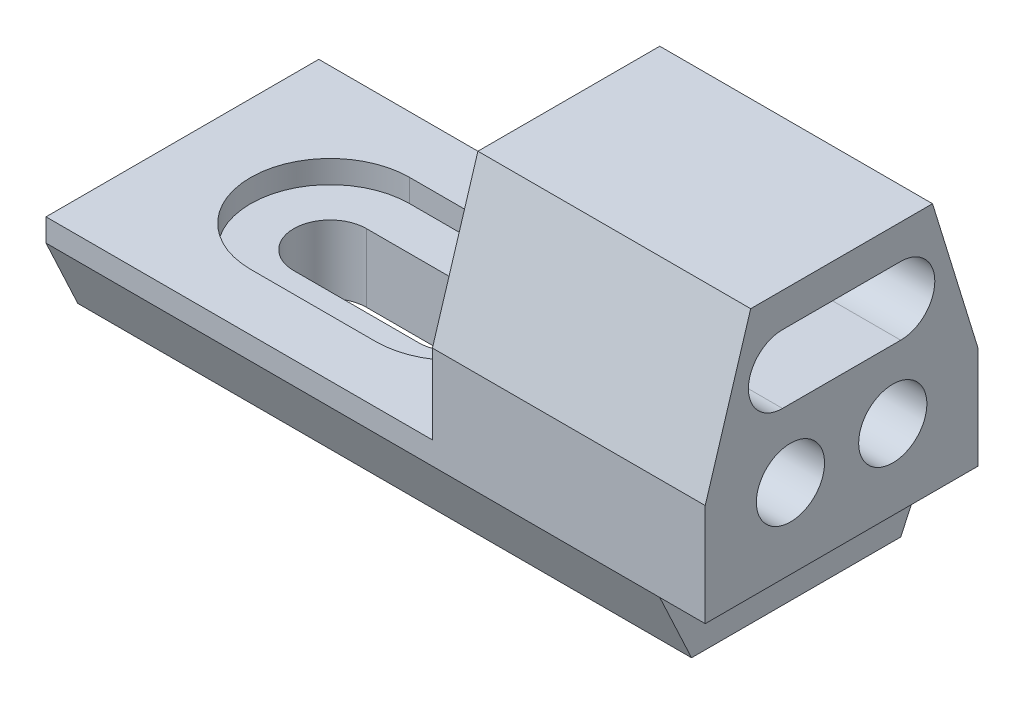
ISO-10303-21;
HEADER;
FILE_DESCRIPTION(('STEP AP214'),'2;1');
FILE_NAME('part.step','',(''),(''),'','','');
FILE_SCHEMA(('AUTOMOTIVE_DESIGN { 1 0 10303 214 1 1 1 1 }'));
ENDSEC;
DATA;
#1=APPLICATION_CONTEXT('core data for automotive mechanical design processes');
#2=APPLICATION_PROTOCOL_DEFINITION('international standard','automotive_design',2000,#1);
#3=PRODUCT_CONTEXT('',#1,'mechanical');
#4=PRODUCT('Part','Part','',(#3));
#5=PRODUCT_RELATED_PRODUCT_CATEGORY('part','',(#4));
#6=PRODUCT_DEFINITION_FORMATION('','',#4);
#7=PRODUCT_DEFINITION_CONTEXT('part definition',#1,'design');
#8=PRODUCT_DEFINITION('design','',#6,#7);
#9=PRODUCT_DEFINITION_SHAPE('','',#8);
#10=(LENGTH_UNIT() NAMED_UNIT(*) SI_UNIT(.MILLI.,.METRE.));
#11=(NAMED_UNIT(*) PLANE_ANGLE_UNIT() SI_UNIT($,.RADIAN.));
#12=(NAMED_UNIT(*) SI_UNIT($,.STERADIAN.) SOLID_ANGLE_UNIT());
#13=UNCERTAINTY_MEASURE_WITH_UNIT(LENGTH_MEASURE(1.E-05),#10,'distance_accuracy_value','');
#14=(GEOMETRIC_REPRESENTATION_CONTEXT(3) GLOBAL_UNCERTAINTY_ASSIGNED_CONTEXT((#13)) GLOBAL_UNIT_ASSIGNED_CONTEXT((#10,
#11,#12)) REPRESENTATION_CONTEXT('',''));
#15=CARTESIAN_POINT('',(0.,0.,0.));
#16=DIRECTION('',(0.,0.,1.));
#17=DIRECTION('',(1.,0.,0.));
#18=AXIS2_PLACEMENT_3D('',#15,#16,#17);
#19=CARTESIAN_POINT('',(0.,10.,0.));
#20=DIRECTION('',(0.,1.,0.));
#21=DIRECTION('',(0.,0.,1.));
#22=AXIS2_PLACEMENT_3D('',#19,#20,#21);
#23=PLANE('',#22);
#24=CARTESIAN_POINT('',(-80.,10.,0.));
#25=DIRECTION('',(0.,1.,0.));
#26=DIRECTION('',(0.,0.,1.));
#27=AXIS2_PLACEMENT_3D('',#24,#25,#26);
#28=CIRCLE('',#27,35.);
#29=CARTESIAN_POINT('',(-80.,10.,-35.));
#30=VERTEX_POINT('',#29);
#31=CARTESIAN_POINT('',(-80.,10.,35.));
#32=VERTEX_POINT('',#31);
#33=EDGE_CURVE('E222',#30,#32,#28,.T.);
#34=ORIENTED_EDGE('',*,*,#33,.F.);
#35=DIRECTION('',(-1.,0.,0.));
#36=VECTOR('',#35,1.);
#37=CARTESIAN_POINT('',(-80.,10.,-35.));
#38=LINE('',#37,#36);
#39=CARTESIAN_POINT('',(-25.,10.,-35.));
#40=VERTEX_POINT('',#39);
#41=EDGE_CURVE('E228',#40,#30,#38,.T.);
#42=ORIENTED_EDGE('',*,*,#41,.F.);
#43=CARTESIAN_POINT('',(-25.,10.,0.));
#44=DIRECTION('',(0.,1.,0.));
#45=DIRECTION('',(0.,0.,1.));
#46=AXIS2_PLACEMENT_3D('',#43,#44,#45);
#47=CIRCLE('',#46,35.);
#48=CARTESIAN_POINT('',(-25.,10.,35.));
#49=VERTEX_POINT('',#48);
#50=EDGE_CURVE('E244',#49,#40,#47,.T.);
#51=ORIENTED_EDGE('',*,*,#50,.F.);
#52=DIRECTION('',(1.,0.,0.));
#53=VECTOR('',#52,1.);
#54=CARTESIAN_POINT('',(-80.,10.,35.));
#55=LINE('',#54,#53);
#56=EDGE_CURVE('E238',#32,#49,#55,.T.);
#57=ORIENTED_EDGE('',*,*,#56,.F.);
#58=EDGE_LOOP('',(#34,#42,#51,#57));
#59=FACE_BOUND('',#58,.T.);
#60=DIRECTION('',(1.,0.,0.));
#61=VECTOR('',#60,1.);
#62=CARTESIAN_POINT('',(-145.,10.,60.));
#63=LINE('',#62,#61);
#64=CARTESIAN_POINT('',(-145.,10.,60.));
#65=VERTEX_POINT('',#64);
#66=CARTESIAN_POINT('',(25.,10.,60.));
#67=VERTEX_POINT('',#66);
#68=EDGE_CURVE('E366',#65,#67,#63,.T.);
#69=ORIENTED_EDGE('',*,*,#68,.T.);
#70=DIRECTION('',(0.,0.,-1.));
#71=VECTOR('',#70,1.);
#72=CARTESIAN_POINT('',(25.,10.,60.));
#73=LINE('',#72,#71);
#74=CARTESIAN_POINT('',(25.,10.,-60.));
#75=VERTEX_POINT('',#74);
#76=EDGE_CURVE('E312',#67,#75,#73,.T.);
#77=ORIENTED_EDGE('',*,*,#76,.T.);
#78=DIRECTION('',(-1.,0.,0.));
#79=VECTOR('',#78,1.);
#80=CARTESIAN_POINT('',(145.,10.,-60.));
#81=LINE('',#80,#79);
#82=CARTESIAN_POINT('',(-145.,10.,-60.));
#83=VERTEX_POINT('',#82);
#84=EDGE_CURVE('E361',#75,#83,#81,.T.);
#85=ORIENTED_EDGE('',*,*,#84,.T.);
#86=DIRECTION('',(0.,0.,1.));
#87=VECTOR('',#86,1.);
#88=CARTESIAN_POINT('',(-145.,10.,-60.));
#89=LINE('',#88,#87);
#90=EDGE_CURVE('E364',#83,#65,#89,.T.);
#91=ORIENTED_EDGE('',*,*,#90,.T.);
#92=EDGE_LOOP('',(#69,#77,#85,#91));
#93=FACE_BOUND('',#92,.T.);
#94=ADVANCED_FACE('F41',(#59,#93),#23,.T.);
#95=CARTESIAN_POINT('',(145.,10.,0.));
#96=DIRECTION('',(-1.,0.,0.));
#97=DIRECTION('',(0.,0.,1.));
#98=AXIS2_PLACEMENT_3D('',#95,#96,#97);
#99=PLANE('',#98);
#100=DIRECTION('',(0.,0.,-1.));
#101=VECTOR('',#100,1.);
#102=CARTESIAN_POINT('',(145.,95.,0.));
#103=LINE('',#102,#101);
#104=CARTESIAN_POINT('',(145.,95.,26.));
#105=VERTEX_POINT('',#104);
#106=CARTESIAN_POINT('',(145.,95.,-26.));
#107=VERTEX_POINT('',#106);
#108=EDGE_CURVE('E294',#105,#107,#103,.T.);
#109=ORIENTED_EDGE('',*,*,#108,.T.);
#110=CARTESIAN_POINT('',(145.,80.,-26.));
#111=DIRECTION('',(-1.,0.,0.));
#112=DIRECTION('',(0.,0.,1.));
#113=AXIS2_PLACEMENT_3D('',#110,#111,#112);
#114=CIRCLE('',#113,15.);
#115=CARTESIAN_POINT('',(145.,65.,-26.));
#116=VERTEX_POINT('',#115);
#117=EDGE_CURVE('E297',#107,#116,#114,.T.);
#118=ORIENTED_EDGE('',*,*,#117,.T.);
#119=DIRECTION('',(0.,0.,1.));
#120=VECTOR('',#119,1.);
#121=CARTESIAN_POINT('',(145.,65.,0.));
#122=LINE('',#121,#120);
#123=CARTESIAN_POINT('',(145.,65.,26.));
#124=VERTEX_POINT('',#123);
#125=EDGE_CURVE('E287',#116,#124,#122,.T.);
#126=ORIENTED_EDGE('',*,*,#125,.T.);
#127=CARTESIAN_POINT('',(145.,80.,26.));
#128=DIRECTION('',(-1.,0.,0.));
#129=DIRECTION('',(0.,0.,1.));
#130=AXIS2_PLACEMENT_3D('',#127,#128,#129);
#131=CIRCLE('',#130,15.);
#132=EDGE_CURVE('E292',#124,#105,#131,.T.);
#133=ORIENTED_EDGE('',*,*,#132,.T.);
#134=EDGE_LOOP('',(#109,#118,#126,#133));
#135=FACE_BOUND('',#134,.T.);
#136=CARTESIAN_POINT('',(145.,35.,22.5));
#137=DIRECTION('',(-1.,0.,0.));
#138=DIRECTION('',(0.,0.,1.));
#139=AXIS2_PLACEMENT_3D('',#136,#137,#138);
#140=CIRCLE('',#139,15.);
#141=CARTESIAN_POINT('',(145.,35.,37.5));
#142=VERTEX_POINT('',#141);
#143=EDGE_CURVE('E285',#142,#142,#140,.T.);
#144=ORIENTED_EDGE('',*,*,#143,.T.);
#145=EDGE_LOOP('',(#144));
#146=FACE_BOUND('',#145,.T.);
#147=CARTESIAN_POINT('',(145.,35.,-22.5));
#148=DIRECTION('',(-1.,0.,0.));
#149=DIRECTION('',(0.,0.,1.));
#150=AXIS2_PLACEMENT_3D('',#147,#148,#149);
#151=CIRCLE('',#150,15.);
#152=CARTESIAN_POINT('',(145.,35.,-7.5));
#153=VERTEX_POINT('',#152);
#154=EDGE_CURVE('E275',#153,#153,#151,.T.);
#155=ORIENTED_EDGE('',*,*,#154,.T.);
#156=EDGE_LOOP('',(#155));
#157=FACE_BOUND('',#156,.T.);
#158=DIRECTION('',(0.,0.,-1.));
#159=VECTOR('',#158,1.);
#160=CARTESIAN_POINT('',(145.,0.,0.));
#161=LINE('',#160,#159);
#162=CARTESIAN_POINT('',(145.,0.,60.));
#163=VERTEX_POINT('',#162);
#164=CARTESIAN_POINT('',(145.,0.,-60.));
#165=VERTEX_POINT('',#164);
#166=EDGE_CURVE('E357',#163,#165,#161,.T.);
#167=ORIENTED_EDGE('',*,*,#166,.T.);
#168=DIRECTION('',(0.,-1.,0.));
#169=VECTOR('',#168,1.);
#170=CARTESIAN_POINT('',(145.,10.,-60.));
#171=LINE('',#170,#169);
#172=CARTESIAN_POINT('',(145.,45.,-60.));
#173=VERTEX_POINT('',#172);
#174=EDGE_CURVE('E390',#173,#165,#171,.T.);
#175=ORIENTED_EDGE('',*,*,#174,.F.);
#176=DIRECTION('',(0.,0.95577900872195,0.294085848837523));
#177=VECTOR('',#176,1.);
#178=CARTESIAN_POINT('',(145.,45.,-60.));
#179=LINE('',#178,#177);
#180=CARTESIAN_POINT('',(145.,110.,-40.));
#181=VERTEX_POINT('',#180);
#182=EDGE_CURVE('E306',#173,#181,#179,.T.);
#183=ORIENTED_EDGE('',*,*,#182,.T.);
#184=DIRECTION('',(0.,0.,1.));
#185=VECTOR('',#184,1.);
#186=CARTESIAN_POINT('',(145.,110.,0.));
#187=LINE('',#186,#185);
#188=CARTESIAN_POINT('',(145.,110.,40.));
#189=VERTEX_POINT('',#188);
#190=EDGE_CURVE('E303',#181,#189,#187,.T.);
#191=ORIENTED_EDGE('',*,*,#190,.T.);
#192=DIRECTION('',(0.,-0.95577900872195,0.294085848837523));
#193=VECTOR('',#192,1.);
#194=CARTESIAN_POINT('',(145.,45.,60.));
#195=LINE('',#194,#193);
#196=CARTESIAN_POINT('',(145.,45.,60.));
#197=VERTEX_POINT('',#196);
#198=EDGE_CURVE('E305',#189,#197,#195,.T.);
#199=ORIENTED_EDGE('',*,*,#198,.T.);
#200=DIRECTION('',(0.,-1.,0.));
#201=VECTOR('',#200,1.);
#202=CARTESIAN_POINT('',(145.,10.,60.));
#203=LINE('',#202,#201);
#204=EDGE_CURVE('E371',#197,#163,#203,.T.);
#205=ORIENTED_EDGE('',*,*,#204,.T.);
#206=EDGE_LOOP('',(#167,#175,#183,#191,#199,#205));
#207=FACE_BOUND('',#206,.T.);
#208=ADVANCED_FACE('F43',(#135,#146,#157,#207),#99,.F.);
#209=CARTESIAN_POINT('',(145.,10.,-60.));
#210=DIRECTION('',(0.,0.,1.));
#211=DIRECTION('',(1.,0.,0.));
#212=AXIS2_PLACEMENT_3D('',#209,#210,#211);
#213=PLANE('',#212);
#214=DIRECTION('',(-1.,0.,0.));
#215=VECTOR('',#214,1.);
#216=CARTESIAN_POINT('',(145.,0.,-60.));
#217=LINE('',#216,#215);
#218=CARTESIAN_POINT('',(125.,0.,-60.));
#219=VERTEX_POINT('',#218);
#220=EDGE_CURVE('E373',#165,#219,#217,.T.);
#221=ORIENTED_EDGE('',*,*,#220,.T.);
#222=DIRECTION('',(-1.,0.,0.));
#223=VECTOR('',#222,1.);
#224=CARTESIAN_POINT('',(125.,0.,-60.));
#225=LINE('',#224,#223);
#226=CARTESIAN_POINT('',(-145.,0.,-60.));
#227=VERTEX_POINT('',#226);
#228=EDGE_CURVE('E360',#219,#227,#225,.T.);
#229=ORIENTED_EDGE('',*,*,#228,.T.);
#230=DIRECTION('',(0.,-1.,0.));
#231=VECTOR('',#230,1.);
#232=CARTESIAN_POINT('',(-145.,10.,-60.));
#233=LINE('',#232,#231);
#234=EDGE_CURVE('E383',#83,#227,#233,.T.);
#235=ORIENTED_EDGE('',*,*,#234,.F.);
#236=ORIENTED_EDGE('',*,*,#84,.F.);
#237=DIRECTION('',(0.,1.,0.));
#238=VECTOR('',#237,1.);
#239=CARTESIAN_POINT('',(25.,10.,-60.));
#240=LINE('',#239,#238);
#241=CARTESIAN_POINT('',(25.,45.,-60.));
#242=VERTEX_POINT('',#241);
#243=EDGE_CURVE('E318',#75,#242,#240,.T.);
#244=ORIENTED_EDGE('',*,*,#243,.T.);
#245=DIRECTION('',(-1.,0.,0.));
#246=VECTOR('',#245,1.);
#247=CARTESIAN_POINT('',(145.,45.,-60.));
#248=LINE('',#247,#246);
#249=EDGE_CURVE('E324',#173,#242,#248,.T.);
#250=ORIENTED_EDGE('',*,*,#249,.F.);
#251=ORIENTED_EDGE('',*,*,#174,.T.);
#252=EDGE_LOOP('',(#221,#229,#235,#236,#244,#250,#251));
#253=FACE_BOUND('',#252,.T.);
#254=ADVANCED_FACE('F415',(#253),#213,.F.);
#255=CARTESIAN_POINT('',(-145.,10.,-60.));
#256=DIRECTION('',(1.,0.,0.));
#257=DIRECTION('',(0.,0.,-1.));
#258=AXIS2_PLACEMENT_3D('',#255,#256,#257);
#259=PLANE('',#258);
#260=ORIENTED_EDGE('',*,*,#234,.T.);
#261=DIRECTION('',(0.,-0.906307787036651,0.422618261740697));
#262=VECTOR('',#261,1.);
#263=CARTESIAN_POINT('',(-145.,0.,-60.));
#264=LINE('',#263,#262);
#265=CARTESIAN_POINT('',(-145.,-30.,-46.0107702553501));
#266=VERTEX_POINT('',#265);
#267=EDGE_CURVE('E338',#227,#266,#264,.T.);
#268=ORIENTED_EDGE('',*,*,#267,.T.);
#269=DIRECTION('',(0.,0.,1.));
#270=VECTOR('',#269,1.);
#271=CARTESIAN_POINT('',(-145.,-30.,46.0107702553502));
#272=LINE('',#271,#270);
#273=CARTESIAN_POINT('',(-145.,-30.,46.0107702553502));
#274=VERTEX_POINT('',#273);
#275=EDGE_CURVE('E331',#266,#274,#272,.T.);
#276=ORIENTED_EDGE('',*,*,#275,.T.);
#277=DIRECTION('',(0.,0.906307787036651,0.422618261740696));
#278=VECTOR('',#277,1.);
#279=CARTESIAN_POINT('',(-145.,0.,60.));
#280=LINE('',#279,#278);
#281=CARTESIAN_POINT('',(-145.,0.,60.));
#282=VERTEX_POINT('',#281);
#283=EDGE_CURVE('E351',#274,#282,#280,.T.);
#284=ORIENTED_EDGE('',*,*,#283,.T.);
#285=DIRECTION('',(0.,-1.,0.));
#286=VECTOR('',#285,1.);
#287=CARTESIAN_POINT('',(-145.,10.,60.));
#288=LINE('',#287,#286);
#289=EDGE_CURVE('E381',#65,#282,#288,.T.);
#290=ORIENTED_EDGE('',*,*,#289,.F.);
#291=ORIENTED_EDGE('',*,*,#90,.F.);
#292=EDGE_LOOP('',(#260,#268,#276,#284,#290,#291));
#293=FACE_BOUND('',#292,.T.);
#294=ADVANCED_FACE('F409',(#293),#259,.F.);
#295=CARTESIAN_POINT('',(-145.,10.,60.));
#296=DIRECTION('',(0.,0.,-1.));
#297=DIRECTION('',(-1.,0.,0.));
#298=AXIS2_PLACEMENT_3D('',#295,#296,#297);
#299=PLANE('',#298);
#300=DIRECTION('',(1.,0.,0.));
#301=VECTOR('',#300,1.);
#302=CARTESIAN_POINT('',(-145.,0.,60.));
#303=LINE('',#302,#301);
#304=CARTESIAN_POINT('',(125.,0.,60.));
#305=VERTEX_POINT('',#304);
#306=EDGE_CURVE('E368',#282,#305,#303,.T.);
#307=ORIENTED_EDGE('',*,*,#306,.T.);
#308=EDGE_CURVE('E376',#305,#163,#303,.T.);
#309=ORIENTED_EDGE('',*,*,#308,.T.);
#310=ORIENTED_EDGE('',*,*,#204,.F.);
#311=DIRECTION('',(-1.,0.,0.));
#312=VECTOR('',#311,1.);
#313=CARTESIAN_POINT('',(145.,45.,60.));
#314=LINE('',#313,#312);
#315=CARTESIAN_POINT('',(25.,45.,60.));
#316=VERTEX_POINT('',#315);
#317=EDGE_CURVE('E327',#197,#316,#314,.T.);
#318=ORIENTED_EDGE('',*,*,#317,.T.);
#319=DIRECTION('',(0.,-1.,0.));
#320=VECTOR('',#319,1.);
#321=CARTESIAN_POINT('',(25.,10.,60.));
#322=LINE('',#321,#320);
#323=EDGE_CURVE('E311',#316,#67,#322,.T.);
#324=ORIENTED_EDGE('',*,*,#323,.T.);
#325=ORIENTED_EDGE('',*,*,#68,.F.);
#326=ORIENTED_EDGE('',*,*,#289,.T.);
#327=EDGE_LOOP('',(#307,#309,#310,#318,#324,#325,#326));
#328=FACE_BOUND('',#327,.T.);
#329=ADVANCED_FACE('F427',(#328),#299,.F.);
#330=CARTESIAN_POINT('',(0.,0.,0.));
#331=DIRECTION('',(0.,1.,0.));
#332=DIRECTION('',(0.,0.,1.));
#333=AXIS2_PLACEMENT_3D('',#330,#331,#332);
#334=PLANE('',#333);
#335=ORIENTED_EDGE('',*,*,#308,.F.);
#336=DIRECTION('',(0.,0.,-1.));
#337=VECTOR('',#336,1.);
#338=CARTESIAN_POINT('',(125.,0.,-60.));
#339=LINE('',#338,#337);
#340=EDGE_CURVE('E344',#305,#219,#339,.T.);
#341=ORIENTED_EDGE('',*,*,#340,.T.);
#342=ORIENTED_EDGE('',*,*,#220,.F.);
#343=ORIENTED_EDGE('',*,*,#166,.F.);
#344=EDGE_LOOP('',(#335,#341,#342,#343));
#345=FACE_BOUND('',#344,.T.);
#346=ADVANCED_FACE('F405',(#345),#334,.F.);
#347=CARTESIAN_POINT('',(125.,-30.,46.0107702553501));
#348=DIRECTION('',(0.,-1.,0.));
#349=DIRECTION('',(0.,0.,-1.));
#350=AXIS2_PLACEMENT_3D('',#347,#348,#349);
#351=PLANE('',#350);
#352=CARTESIAN_POINT('',(-80.,-30.,0.));
#353=DIRECTION('',(0.,-1.,0.));
#354=DIRECTION('',(0.,0.,-1.));
#355=AXIS2_PLACEMENT_3D('',#352,#353,#354);
#356=CIRCLE('',#355,16.);
#357=CARTESIAN_POINT('',(-80.,-30.,16.));
#358=VERTEX_POINT('',#357);
#359=CARTESIAN_POINT('',(-80.,-30.,-16.));
#360=VERTEX_POINT('',#359);
#361=EDGE_CURVE('E11',#358,#360,#356,.T.);
#362=ORIENTED_EDGE('',*,*,#361,.F.);
#363=DIRECTION('',(-1.,0.,0.));
#364=VECTOR('',#363,1.);
#365=CARTESIAN_POINT('',(125.,-30.,16.));
#366=LINE('',#365,#364);
#367=CARTESIAN_POINT('',(-25.,-30.,16.));
#368=VERTEX_POINT('',#367);
#369=EDGE_CURVE('E199',#368,#358,#366,.T.);
#370=ORIENTED_EDGE('',*,*,#369,.F.);
#371=CARTESIAN_POINT('',(-25.,-30.,0.));
#372=DIRECTION('',(0.,-1.,0.));
#373=DIRECTION('',(0.,0.,-1.));
#374=AXIS2_PLACEMENT_3D('',#371,#372,#373);
#375=CIRCLE('',#374,16.);
#376=CARTESIAN_POINT('',(-25.,-30.,-16.));
#377=VERTEX_POINT('',#376);
#378=EDGE_CURVE('E391',#377,#368,#375,.T.);
#379=ORIENTED_EDGE('',*,*,#378,.F.);
#380=DIRECTION('',(1.,0.,0.));
#381=VECTOR('',#380,1.);
#382=CARTESIAN_POINT('',(125.,-30.,-16.));
#383=LINE('',#382,#381);
#384=EDGE_CURVE('E47',#360,#377,#383,.T.);
#385=ORIENTED_EDGE('',*,*,#384,.F.);
#386=EDGE_LOOP('',(#362,#370,#379,#385));
#387=FACE_BOUND('',#386,.T.);
#388=ORIENTED_EDGE('',*,*,#275,.F.);
#389=DIRECTION('',(-1.,0.,0.));
#390=VECTOR('',#389,1.);
#391=CARTESIAN_POINT('',(125.,-30.,-46.0107702553502));
#392=LINE('',#391,#390);
#393=CARTESIAN_POINT('',(125.,-30.,-46.0107702553502));
#394=VERTEX_POINT('',#393);
#395=EDGE_CURVE('E358',#394,#266,#392,.T.);
#396=ORIENTED_EDGE('',*,*,#395,.F.);
#397=DIRECTION('',(0.,0.,1.));
#398=VECTOR('',#397,1.);
#399=CARTESIAN_POINT('',(125.,-30.,46.0107702553501));
#400=LINE('',#399,#398);
#401=CARTESIAN_POINT('',(125.,-30.,46.0107702553501));
#402=VERTEX_POINT('',#401);
#403=EDGE_CURVE('E333',#394,#402,#400,.T.);
#404=ORIENTED_EDGE('',*,*,#403,.T.);
#405=DIRECTION('',(-1.,0.,0.));
#406=VECTOR('',#405,1.);
#407=CARTESIAN_POINT('',(125.,-30.,46.0107702553501));
#408=LINE('',#407,#406);
#409=EDGE_CURVE('E346',#402,#274,#408,.T.);
#410=ORIENTED_EDGE('',*,*,#409,.T.);
#411=EDGE_LOOP('',(#388,#396,#404,#410));
#412=FACE_BOUND('',#411,.T.);
#413=ADVANCED_FACE('F397',(#387,#412),#351,.T.);
#414=CARTESIAN_POINT('',(125.,0.,-60.));
#415=DIRECTION('',(0.,-0.422618261740697,-0.906307787036651));
#416=DIRECTION('',(0.,0.906307787036651,-0.422618261740697));
#417=AXIS2_PLACEMENT_3D('',#414,#415,#416);
#418=PLANE('',#417);
#419=ORIENTED_EDGE('',*,*,#267,.F.);
#420=ORIENTED_EDGE('',*,*,#228,.F.);
#421=DIRECTION('',(0.,-0.906307787036651,0.422618261740697));
#422=VECTOR('',#421,1.);
#423=CARTESIAN_POINT('',(125.,0.,-60.));
#424=LINE('',#423,#422);
#425=EDGE_CURVE('E341',#219,#394,#424,.T.);
#426=ORIENTED_EDGE('',*,*,#425,.T.);
#427=ORIENTED_EDGE('',*,*,#395,.T.);
#428=EDGE_LOOP('',(#419,#420,#426,#427));
#429=FACE_BOUND('',#428,.T.);
#430=ADVANCED_FACE('F402',(#429),#418,.T.);
#431=CARTESIAN_POINT('',(125.,0.,60.));
#432=DIRECTION('',(0.,-0.422618261740696,0.906307787036651));
#433=DIRECTION('',(0.,-0.906307787036652,-0.422618261740696));
#434=AXIS2_PLACEMENT_3D('',#431,#432,#433);
#435=PLANE('',#434);
#436=ORIENTED_EDGE('',*,*,#283,.F.);
#437=ORIENTED_EDGE('',*,*,#409,.F.);
#438=DIRECTION('',(0.,0.906307787036651,0.422618261740696));
#439=VECTOR('',#438,1.);
#440=CARTESIAN_POINT('',(125.,0.,60.));
#441=LINE('',#440,#439);
#442=EDGE_CURVE('E339',#402,#305,#441,.T.);
#443=ORIENTED_EDGE('',*,*,#442,.T.);
#444=ORIENTED_EDGE('',*,*,#306,.F.);
#445=EDGE_LOOP('',(#436,#437,#443,#444));
#446=FACE_BOUND('',#445,.T.);
#447=ADVANCED_FACE('F422',(#446),#435,.T.);
#448=CARTESIAN_POINT('',(125.,-1.34151948808873E-13,0.));
#449=DIRECTION('',(-1.,0.,0.));
#450=DIRECTION('',(0.,-1.,0.));
#451=AXIS2_PLACEMENT_3D('',#448,#449,#450);
#452=PLANE('',#451);
#453=ORIENTED_EDGE('',*,*,#403,.F.);
#454=ORIENTED_EDGE('',*,*,#425,.F.);
#455=ORIENTED_EDGE('',*,*,#340,.F.);
#456=ORIENTED_EDGE('',*,*,#442,.F.);
#457=EDGE_LOOP('',(#453,#454,#455,#456));
#458=FACE_BOUND('',#457,.T.);
#459=ADVANCED_FACE('F421',(#458),#452,.F.);
#460=CARTESIAN_POINT('',(145.,45.,60.));
#461=DIRECTION('',(0.,-0.294085848837523,-0.95577900872195));
#462=DIRECTION('',(0.,0.95577900872195,-0.294085848837523));
#463=AXIS2_PLACEMENT_3D('',#460,#461,#462);
#464=PLANE('',#463);
#465=DIRECTION('',(0.,-0.95577900872195,0.294085848837523));
#466=VECTOR('',#465,1.);
#467=CARTESIAN_POINT('',(25.,45.,60.));
#468=LINE('',#467,#466);
#469=CARTESIAN_POINT('',(25.,110.,40.));
#470=VERTEX_POINT('',#469);
#471=EDGE_CURVE('E300',#470,#316,#468,.T.);
#472=ORIENTED_EDGE('',*,*,#471,.T.);
#473=ORIENTED_EDGE('',*,*,#317,.F.);
#474=ORIENTED_EDGE('',*,*,#198,.F.);
#475=DIRECTION('',(-1.,0.,0.));
#476=VECTOR('',#475,1.);
#477=CARTESIAN_POINT('',(145.,110.,40.));
#478=LINE('',#477,#476);
#479=EDGE_CURVE('E332',#189,#470,#478,.T.);
#480=ORIENTED_EDGE('',*,*,#479,.T.);
#481=EDGE_LOOP('',(#472,#473,#474,#480));
#482=FACE_BOUND('',#481,.T.);
#483=ADVANCED_FACE('F449',(#482),#464,.F.);
#484=CARTESIAN_POINT('',(145.,45.,-60.));
#485=DIRECTION('',(0.,-0.294085848837523,0.95577900872195));
#486=DIRECTION('',(0.,-0.95577900872195,-0.294085848837523));
#487=AXIS2_PLACEMENT_3D('',#484,#485,#486);
#488=PLANE('',#487);
#489=DIRECTION('',(0.,0.95577900872195,0.294085848837523));
#490=VECTOR('',#489,1.);
#491=CARTESIAN_POINT('',(25.,45.,-60.));
#492=LINE('',#491,#490);
#493=CARTESIAN_POINT('',(25.,110.,-40.));
#494=VERTEX_POINT('',#493);
#495=EDGE_CURVE('E319',#242,#494,#492,.T.);
#496=ORIENTED_EDGE('',*,*,#495,.T.);
#497=DIRECTION('',(-1.,0.,0.));
#498=VECTOR('',#497,1.);
#499=CARTESIAN_POINT('',(145.,110.,-40.));
#500=LINE('',#499,#498);
#501=EDGE_CURVE('E313',#181,#494,#500,.T.);
#502=ORIENTED_EDGE('',*,*,#501,.F.);
#503=ORIENTED_EDGE('',*,*,#182,.F.);
#504=ORIENTED_EDGE('',*,*,#249,.T.);
#505=EDGE_LOOP('',(#496,#502,#503,#504));
#506=FACE_BOUND('',#505,.T.);
#507=ADVANCED_FACE('F440',(#506),#488,.F.);
#508=CARTESIAN_POINT('',(145.,110.,0.));
#509=DIRECTION('',(0.,-1.,0.));
#510=DIRECTION('',(0.,0.,-1.));
#511=AXIS2_PLACEMENT_3D('',#508,#509,#510);
#512=PLANE('',#511);
#513=DIRECTION('',(0.,0.,1.));
#514=VECTOR('',#513,1.);
#515=CARTESIAN_POINT('',(25.,110.,0.));
#516=LINE('',#515,#514);
#517=EDGE_CURVE('E301',#494,#470,#516,.T.);
#518=ORIENTED_EDGE('',*,*,#517,.T.);
#519=ORIENTED_EDGE('',*,*,#479,.F.);
#520=ORIENTED_EDGE('',*,*,#190,.F.);
#521=ORIENTED_EDGE('',*,*,#501,.T.);
#522=EDGE_LOOP('',(#518,#519,#520,#521));
#523=FACE_BOUND('',#522,.T.);
#524=ADVANCED_FACE('F441',(#523),#512,.F.);
#525=CARTESIAN_POINT('',(25.,0.,0.));
#526=DIRECTION('',(-1.,0.,0.));
#527=DIRECTION('',(0.,0.,1.));
#528=AXIS2_PLACEMENT_3D('',#525,#526,#527);
#529=PLANE('',#528);
#530=CARTESIAN_POINT('',(25.,80.,-26.));
#531=DIRECTION('',(-1.,0.,0.));
#532=DIRECTION('',(0.,0.,1.));
#533=AXIS2_PLACEMENT_3D('',#530,#531,#532);
#534=CIRCLE('',#533,15.);
#535=CARTESIAN_POINT('',(25.,95.,-26.));
#536=VERTEX_POINT('',#535);
#537=CARTESIAN_POINT('',(25.,65.,-26.));
#538=VERTEX_POINT('',#537);
#539=EDGE_CURVE('E260',#536,#538,#534,.T.);
#540=ORIENTED_EDGE('',*,*,#539,.F.);
#541=DIRECTION('',(0.,0.,-1.));
#542=VECTOR('',#541,1.);
#543=CARTESIAN_POINT('',(25.,95.,-26.));
#544=LINE('',#543,#542);
#545=CARTESIAN_POINT('',(25.,95.,26.));
#546=VERTEX_POINT('',#545);
#547=EDGE_CURVE('E266',#546,#536,#544,.T.);
#548=ORIENTED_EDGE('',*,*,#547,.F.);
#549=CARTESIAN_POINT('',(25.,80.,26.));
#550=DIRECTION('',(-1.,0.,0.));
#551=DIRECTION('',(0.,0.,1.));
#552=AXIS2_PLACEMENT_3D('',#549,#550,#551);
#553=CIRCLE('',#552,15.);
#554=CARTESIAN_POINT('',(25.,65.,26.));
#555=VERTEX_POINT('',#554);
#556=EDGE_CURVE('E263',#555,#546,#553,.T.);
#557=ORIENTED_EDGE('',*,*,#556,.F.);
#558=DIRECTION('',(0.,0.,1.));
#559=VECTOR('',#558,1.);
#560=CARTESIAN_POINT('',(25.,65.,-26.));
#561=LINE('',#560,#559);
#562=EDGE_CURVE('E259',#538,#555,#561,.T.);
#563=ORIENTED_EDGE('',*,*,#562,.F.);
#564=EDGE_LOOP('',(#540,#548,#557,#563));
#565=FACE_BOUND('',#564,.T.);
#566=CARTESIAN_POINT('',(25.,35.,22.5));
#567=DIRECTION('',(-1.,0.,0.));
#568=DIRECTION('',(0.,0.,1.));
#569=AXIS2_PLACEMENT_3D('',#566,#567,#568);
#570=CIRCLE('',#569,15.);
#571=CARTESIAN_POINT('',(25.,35.,37.5));
#572=VERTEX_POINT('',#571);
#573=EDGE_CURVE('E257',#572,#572,#570,.T.);
#574=ORIENTED_EDGE('',*,*,#573,.F.);
#575=EDGE_LOOP('',(#574));
#576=FACE_BOUND('',#575,.T.);
#577=CARTESIAN_POINT('',(25.,35.,-22.5));
#578=DIRECTION('',(-1.,0.,0.));
#579=DIRECTION('',(0.,0.,1.));
#580=AXIS2_PLACEMENT_3D('',#577,#578,#579);
#581=CIRCLE('',#580,15.);
#582=CARTESIAN_POINT('',(25.,35.,-7.5));
#583=VERTEX_POINT('',#582);
#584=EDGE_CURVE('E246',#583,#583,#581,.T.);
#585=ORIENTED_EDGE('',*,*,#584,.F.);
#586=EDGE_LOOP('',(#585));
#587=FACE_BOUND('',#586,.T.);
#588=ORIENTED_EDGE('',*,*,#471,.F.);
#589=ORIENTED_EDGE('',*,*,#517,.F.);
#590=ORIENTED_EDGE('',*,*,#495,.F.);
#591=ORIENTED_EDGE('',*,*,#243,.F.);
#592=ORIENTED_EDGE('',*,*,#76,.F.);
#593=ORIENTED_EDGE('',*,*,#323,.F.);
#594=EDGE_LOOP('',(#588,#589,#590,#591,#592,#593));
#595=FACE_BOUND('',#594,.T.);
#596=ADVANCED_FACE('F442',(#565,#576,#587,#595),#529,.T.);
#597=CARTESIAN_POINT('',(237.,35.,-22.5));
#598=DIRECTION('',(-1.,0.,0.));
#599=DIRECTION('',(0.,0.,1.));
#600=AXIS2_PLACEMENT_3D('',#597,#598,#599);
#601=CYLINDRICAL_SURFACE('',#600,15.);
#602=ORIENTED_EDGE('',*,*,#584,.T.);
#603=EDGE_LOOP('',(#602));
#604=FACE_BOUND('',#603,.T.);
#605=ORIENTED_EDGE('',*,*,#154,.F.);
#606=EDGE_LOOP('',(#605));
#607=FACE_BOUND('',#606,.T.);
#608=ADVANCED_FACE('F523',(#604,#607),#601,.F.);
#609=CARTESIAN_POINT('',(237.,35.,22.5));
#610=DIRECTION('',(-1.,0.,0.));
#611=DIRECTION('',(0.,0.,1.));
#612=AXIS2_PLACEMENT_3D('',#609,#610,#611);
#613=CYLINDRICAL_SURFACE('',#612,15.);
#614=ORIENTED_EDGE('',*,*,#573,.T.);
#615=EDGE_LOOP('',(#614));
#616=FACE_BOUND('',#615,.T.);
#617=ORIENTED_EDGE('',*,*,#143,.F.);
#618=EDGE_LOOP('',(#617));
#619=FACE_BOUND('',#618,.T.);
#620=ADVANCED_FACE('F533',(#616,#619),#613,.F.);
#621=CARTESIAN_POINT('',(237.,80.,-26.));
#622=DIRECTION('',(-1.,0.,0.));
#623=DIRECTION('',(0.,0.,1.));
#624=AXIS2_PLACEMENT_3D('',#621,#622,#623);
#625=CYLINDRICAL_SURFACE('',#624,15.);
#626=DIRECTION('',(-1.,0.,0.));
#627=VECTOR('',#626,1.);
#628=CARTESIAN_POINT('',(237.,95.,-26.));
#629=LINE('',#628,#627);
#630=EDGE_CURVE('E269',#107,#536,#629,.T.);
#631=ORIENTED_EDGE('',*,*,#630,.T.);
#632=ORIENTED_EDGE('',*,*,#539,.T.);
#633=DIRECTION('',(-1.,0.,0.));
#634=VECTOR('',#633,1.);
#635=CARTESIAN_POINT('',(237.,65.,-26.));
#636=LINE('',#635,#634);
#637=EDGE_CURVE('E267',#116,#538,#636,.T.);
#638=ORIENTED_EDGE('',*,*,#637,.F.);
#639=ORIENTED_EDGE('',*,*,#117,.F.);
#640=EDGE_LOOP('',(#631,#632,#638,#639));
#641=FACE_BOUND('',#640,.T.);
#642=ADVANCED_FACE('F541',(#641),#625,.F.);
#643=CARTESIAN_POINT('',(237.,95.,-26.));
#644=DIRECTION('',(0.,1.,0.));
#645=DIRECTION('',(0.,0.,1.));
#646=AXIS2_PLACEMENT_3D('',#643,#644,#645);
#647=PLANE('',#646);
#648=DIRECTION('',(-1.,0.,0.));
#649=VECTOR('',#648,1.);
#650=CARTESIAN_POINT('',(237.,95.,26.));
#651=LINE('',#650,#649);
#652=EDGE_CURVE('E272',#105,#546,#651,.T.);
#653=ORIENTED_EDGE('',*,*,#652,.T.);
#654=ORIENTED_EDGE('',*,*,#547,.T.);
#655=ORIENTED_EDGE('',*,*,#630,.F.);
#656=ORIENTED_EDGE('',*,*,#108,.F.);
#657=EDGE_LOOP('',(#653,#654,#655,#656));
#658=FACE_BOUND('',#657,.T.);
#659=ADVANCED_FACE('F552',(#658),#647,.F.);
#660=CARTESIAN_POINT('',(237.,80.,26.));
#661=DIRECTION('',(-1.,0.,0.));
#662=DIRECTION('',(0.,0.,1.));
#663=AXIS2_PLACEMENT_3D('',#660,#661,#662);
#664=CYLINDRICAL_SURFACE('',#663,15.);
#665=DIRECTION('',(-1.,0.,0.));
#666=VECTOR('',#665,1.);
#667=CARTESIAN_POINT('',(237.,65.,26.));
#668=LINE('',#667,#666);
#669=EDGE_CURVE('E274',#124,#555,#668,.T.);
#670=ORIENTED_EDGE('',*,*,#669,.T.);
#671=ORIENTED_EDGE('',*,*,#556,.T.);
#672=ORIENTED_EDGE('',*,*,#652,.F.);
#673=ORIENTED_EDGE('',*,*,#132,.F.);
#674=EDGE_LOOP('',(#670,#671,#672,#673));
#675=FACE_BOUND('',#674,.T.);
#676=ADVANCED_FACE('F563',(#675),#664,.F.);
#677=CARTESIAN_POINT('',(237.,65.,-26.));
#678=DIRECTION('',(0.,-1.,0.));
#679=DIRECTION('',(0.,0.,-1.));
#680=AXIS2_PLACEMENT_3D('',#677,#678,#679);
#681=PLANE('',#680);
#682=ORIENTED_EDGE('',*,*,#637,.T.);
#683=ORIENTED_EDGE('',*,*,#562,.T.);
#684=ORIENTED_EDGE('',*,*,#669,.F.);
#685=ORIENTED_EDGE('',*,*,#125,.F.);
#686=EDGE_LOOP('',(#682,#683,#684,#685));
#687=FACE_BOUND('',#686,.T.);
#688=ADVANCED_FACE('F571',(#687),#681,.F.);
#689=CARTESIAN_POINT('',(-80.,0.,0.));
#690=DIRECTION('',(0.,1.,0.));
#691=DIRECTION('',(0.,0.,1.));
#692=AXIS2_PLACEMENT_3D('',#689,#690,#691);
#693=CYLINDRICAL_SURFACE('',#692,35.);
#694=ORIENTED_EDGE('',*,*,#33,.T.);
#695=DIRECTION('',(0.,1.,0.));
#696=VECTOR('',#695,1.);
#697=CARTESIAN_POINT('',(-80.,0.,35.));
#698=LINE('',#697,#696);
#699=CARTESIAN_POINT('',(-80.,0.,35.));
#700=VERTEX_POINT('',#699);
#701=EDGE_CURVE('E236',#700,#32,#698,.T.);
#702=ORIENTED_EDGE('',*,*,#701,.F.);
#703=CARTESIAN_POINT('',(-80.,0.,0.));
#704=DIRECTION('',(0.,1.,0.));
#705=DIRECTION('',(0.,0.,1.));
#706=AXIS2_PLACEMENT_3D('',#703,#704,#705);
#707=CIRCLE('',#706,35.);
#708=CARTESIAN_POINT('',(-80.,0.,-35.));
#709=VERTEX_POINT('',#708);
#710=EDGE_CURVE('E223',#709,#700,#707,.T.);
#711=ORIENTED_EDGE('',*,*,#710,.F.);
#712=DIRECTION('',(0.,1.,0.));
#713=VECTOR('',#712,1.);
#714=CARTESIAN_POINT('',(-80.,0.,-35.));
#715=LINE('',#714,#713);
#716=EDGE_CURVE('E247',#709,#30,#715,.T.);
#717=ORIENTED_EDGE('',*,*,#716,.T.);
#718=EDGE_LOOP('',(#694,#702,#711,#717));
#719=FACE_BOUND('',#718,.T.);
#720=ADVANCED_FACE('F576',(#719),#693,.F.);
#721=CARTESIAN_POINT('',(-80.,0.,-35.));
#722=DIRECTION('',(0.,0.,-1.));
#723=DIRECTION('',(-1.,0.,0.));
#724=AXIS2_PLACEMENT_3D('',#721,#722,#723);
#725=PLANE('',#724);
#726=ORIENTED_EDGE('',*,*,#41,.T.);
#727=ORIENTED_EDGE('',*,*,#716,.F.);
#728=DIRECTION('',(-1.,0.,0.));
#729=VECTOR('',#728,1.);
#730=CARTESIAN_POINT('',(-80.,0.,-35.));
#731=LINE('',#730,#729);
#732=CARTESIAN_POINT('',(-25.,0.,-35.));
#733=VERTEX_POINT('',#732);
#734=EDGE_CURVE('E231',#733,#709,#731,.T.);
#735=ORIENTED_EDGE('',*,*,#734,.F.);
#736=DIRECTION('',(0.,1.,0.));
#737=VECTOR('',#736,1.);
#738=CARTESIAN_POINT('',(-25.,0.,-35.));
#739=LINE('',#738,#737);
#740=EDGE_CURVE('E253',#733,#40,#739,.T.);
#741=ORIENTED_EDGE('',*,*,#740,.T.);
#742=EDGE_LOOP('',(#726,#727,#735,#741));
#743=FACE_BOUND('',#742,.T.);
#744=ADVANCED_FACE('F589',(#743),#725,.F.);
#745=CARTESIAN_POINT('',(-25.,0.,0.));
#746=DIRECTION('',(0.,1.,0.));
#747=DIRECTION('',(0.,0.,1.));
#748=AXIS2_PLACEMENT_3D('',#745,#746,#747);
#749=CYLINDRICAL_SURFACE('',#748,35.);
#750=ORIENTED_EDGE('',*,*,#50,.T.);
#751=ORIENTED_EDGE('',*,*,#740,.F.);
#752=CARTESIAN_POINT('',(-25.,0.,0.));
#753=DIRECTION('',(0.,1.,0.));
#754=DIRECTION('',(0.,0.,1.));
#755=AXIS2_PLACEMENT_3D('',#752,#753,#754);
#756=CIRCLE('',#755,35.);
#757=CARTESIAN_POINT('',(-25.,0.,35.));
#758=VERTEX_POINT('',#757);
#759=EDGE_CURVE('E234',#758,#733,#756,.T.);
#760=ORIENTED_EDGE('',*,*,#759,.F.);
#761=DIRECTION('',(0.,1.,0.));
#762=VECTOR('',#761,1.);
#763=CARTESIAN_POINT('',(-25.,0.,35.));
#764=LINE('',#763,#762);
#765=EDGE_CURVE('E251',#758,#49,#764,.T.);
#766=ORIENTED_EDGE('',*,*,#765,.T.);
#767=EDGE_LOOP('',(#750,#751,#760,#766));
#768=FACE_BOUND('',#767,.T.);
#769=ADVANCED_FACE('F597',(#768),#749,.F.);
#770=CARTESIAN_POINT('',(-80.,0.,35.));
#771=DIRECTION('',(0.,0.,1.));
#772=DIRECTION('',(1.,0.,0.));
#773=AXIS2_PLACEMENT_3D('',#770,#771,#772);
#774=PLANE('',#773);
#775=ORIENTED_EDGE('',*,*,#56,.T.);
#776=ORIENTED_EDGE('',*,*,#765,.F.);
#777=DIRECTION('',(1.,0.,0.));
#778=VECTOR('',#777,1.);
#779=CARTESIAN_POINT('',(-80.,0.,35.));
#780=LINE('',#779,#778);
#781=EDGE_CURVE('E229',#700,#758,#780,.T.);
#782=ORIENTED_EDGE('',*,*,#781,.F.);
#783=ORIENTED_EDGE('',*,*,#701,.T.);
#784=EDGE_LOOP('',(#775,#776,#782,#783));
#785=FACE_BOUND('',#784,.T.);
#786=ADVANCED_FACE('F606',(#785),#774,.F.);
#787=CARTESIAN_POINT('',(-80.,0.,0.));
#788=DIRECTION('',(0.,1.,0.));
#789=DIRECTION('',(0.,0.,1.));
#790=AXIS2_PLACEMENT_3D('',#787,#788,#789);
#791=PLANE('',#790);
#792=CARTESIAN_POINT('',(-80.,0.,0.));
#793=DIRECTION('',(0.,1.,0.));
#794=DIRECTION('',(0.,0.,1.));
#795=AXIS2_PLACEMENT_3D('',#792,#793,#794);
#796=CIRCLE('',#795,16.);
#797=CARTESIAN_POINT('',(-80.,0.,-16.));
#798=VERTEX_POINT('',#797);
#799=CARTESIAN_POINT('',(-80.,0.,16.));
#800=VERTEX_POINT('',#799);
#801=EDGE_CURVE('E206',#798,#800,#796,.T.);
#802=ORIENTED_EDGE('',*,*,#801,.F.);
#803=DIRECTION('',(-1.,0.,0.));
#804=VECTOR('',#803,1.);
#805=CARTESIAN_POINT('',(-80.,0.,-16.));
#806=LINE('',#805,#804);
#807=CARTESIAN_POINT('',(-25.,0.,-16.));
#808=VERTEX_POINT('',#807);
#809=EDGE_CURVE('E201',#808,#798,#806,.T.);
#810=ORIENTED_EDGE('',*,*,#809,.F.);
#811=CARTESIAN_POINT('',(-25.,0.,0.));
#812=DIRECTION('',(0.,1.,0.));
#813=DIRECTION('',(0.,0.,1.));
#814=AXIS2_PLACEMENT_3D('',#811,#812,#813);
#815=CIRCLE('',#814,16.);
#816=CARTESIAN_POINT('',(-25.,0.,16.));
#817=VERTEX_POINT('',#816);
#818=EDGE_CURVE('E57',#817,#808,#815,.T.);
#819=ORIENTED_EDGE('',*,*,#818,.F.);
#820=DIRECTION('',(1.,0.,0.));
#821=VECTOR('',#820,1.);
#822=CARTESIAN_POINT('',(-80.,0.,16.));
#823=LINE('',#822,#821);
#824=EDGE_CURVE('E196',#800,#817,#823,.T.);
#825=ORIENTED_EDGE('',*,*,#824,.F.);
#826=EDGE_LOOP('',(#802,#810,#819,#825));
#827=FACE_BOUND('',#826,.T.);
#828=ORIENTED_EDGE('',*,*,#710,.T.);
#829=ORIENTED_EDGE('',*,*,#781,.T.);
#830=ORIENTED_EDGE('',*,*,#759,.T.);
#831=ORIENTED_EDGE('',*,*,#734,.T.);
#832=EDGE_LOOP('',(#828,#829,#830,#831));
#833=FACE_BOUND('',#832,.T.);
#834=ADVANCED_FACE('F212',(#827,#833),#791,.T.);
#835=CARTESIAN_POINT('',(-80.,-68.,0.));
#836=DIRECTION('',(0.,1.,0.));
#837=DIRECTION('',(0.,0.,1.));
#838=AXIS2_PLACEMENT_3D('',#835,#836,#837);
#839=CYLINDRICAL_SURFACE('',#838,16.);
#840=ORIENTED_EDGE('',*,*,#361,.T.);
#841=DIRECTION('',(0.,1.,0.));
#842=VECTOR('',#841,1.);
#843=CARTESIAN_POINT('',(-80.,-68.,-16.));
#844=LINE('',#843,#842);
#845=EDGE_CURVE('E207',#360,#798,#844,.T.);
#846=ORIENTED_EDGE('',*,*,#845,.T.);
#847=ORIENTED_EDGE('',*,*,#801,.T.);
#848=DIRECTION('',(0.,1.,0.));
#849=VECTOR('',#848,1.);
#850=CARTESIAN_POINT('',(-80.,-68.,16.));
#851=LINE('',#850,#849);
#852=EDGE_CURVE('E195',#358,#800,#851,.T.);
#853=ORIENTED_EDGE('',*,*,#852,.F.);
#854=EDGE_LOOP('',(#840,#846,#847,#853));
#855=FACE_BOUND('',#854,.T.);
#856=ADVANCED_FACE('F210',(#855),#839,.F.);
#857=CARTESIAN_POINT('',(-80.,-68.,-16.));
#858=DIRECTION('',(0.,0.,-1.));
#859=DIRECTION('',(-1.,0.,0.));
#860=AXIS2_PLACEMENT_3D('',#857,#858,#859);
#861=PLANE('',#860);
#862=ORIENTED_EDGE('',*,*,#384,.T.);
#863=DIRECTION('',(0.,1.,0.));
#864=VECTOR('',#863,1.);
#865=CARTESIAN_POINT('',(-25.,-68.,-16.));
#866=LINE('',#865,#864);
#867=EDGE_CURVE('E225',#377,#808,#866,.T.);
#868=ORIENTED_EDGE('',*,*,#867,.T.);
#869=ORIENTED_EDGE('',*,*,#809,.T.);
#870=ORIENTED_EDGE('',*,*,#845,.F.);
#871=EDGE_LOOP('',(#862,#868,#869,#870));
#872=FACE_BOUND('',#871,.T.);
#873=ADVANCED_FACE('F393',(#872),#861,.F.);
#874=CARTESIAN_POINT('',(-25.,-68.,0.));
#875=DIRECTION('',(0.,1.,0.));
#876=DIRECTION('',(0.,0.,1.));
#877=AXIS2_PLACEMENT_3D('',#874,#875,#876);
#878=CYLINDRICAL_SURFACE('',#877,16.);
#879=ORIENTED_EDGE('',*,*,#378,.T.);
#880=DIRECTION('',(0.,1.,0.));
#881=VECTOR('',#880,1.);
#882=CARTESIAN_POINT('',(-25.,-68.,16.));
#883=LINE('',#882,#881);
#884=EDGE_CURVE('E64',#368,#817,#883,.T.);
#885=ORIENTED_EDGE('',*,*,#884,.T.);
#886=ORIENTED_EDGE('',*,*,#818,.T.);
#887=ORIENTED_EDGE('',*,*,#867,.F.);
#888=EDGE_LOOP('',(#879,#885,#886,#887));
#889=FACE_BOUND('',#888,.T.);
#890=ADVANCED_FACE('F399',(#889),#878,.F.);
#891=CARTESIAN_POINT('',(-80.,-68.,16.));
#892=DIRECTION('',(0.,0.,1.));
#893=DIRECTION('',(1.,0.,0.));
#894=AXIS2_PLACEMENT_3D('',#891,#892,#893);
#895=PLANE('',#894);
#896=ORIENTED_EDGE('',*,*,#369,.T.);
#897=ORIENTED_EDGE('',*,*,#852,.T.);
#898=ORIENTED_EDGE('',*,*,#824,.T.);
#899=ORIENTED_EDGE('',*,*,#884,.F.);
#900=EDGE_LOOP('',(#896,#897,#898,#899));
#901=FACE_BOUND('',#900,.T.);
#902=ADVANCED_FACE('F198',(#901),#895,.F.);
#903=CLOSED_SHELL('',(#94,#208,#254,#294,#329,#346,#413,#430,#447,#459,#483,#507,#524,#596,#608,
#620,#642,#659,#676,#688,#720,#744,#769,#786,#834,#856,#873,#890,#902));
#904=MANIFOLD_SOLID_BREP('B2',#903);
#905=ADVANCED_BREP_SHAPE_REPRESENTATION('',(#18,#904),#14);
#906=SHAPE_DEFINITION_REPRESENTATION(#9,#905);
ENDSEC;
END-ISO-10303-21;
